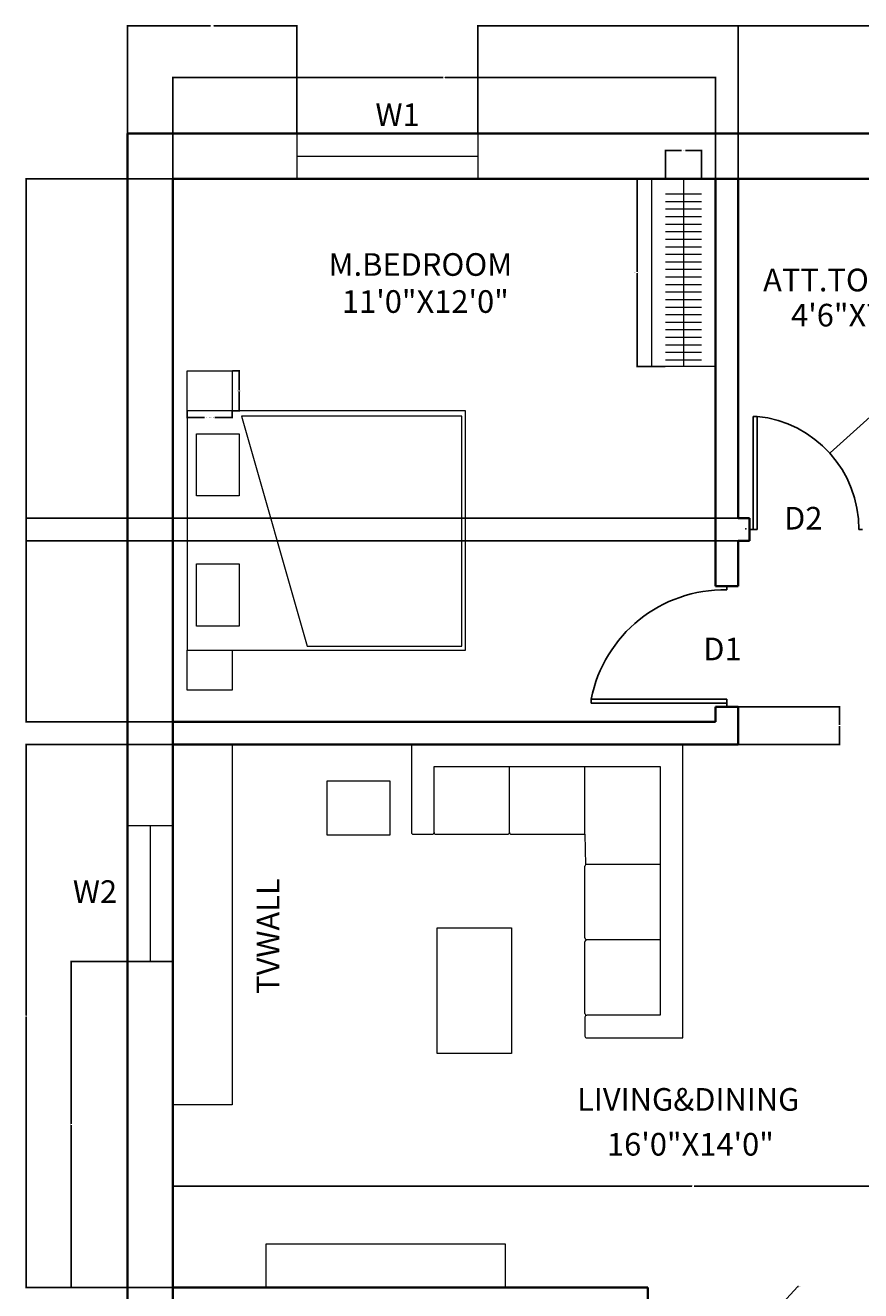
# Model space of a CAD drawing. Units: inches. Extents: x 2906 to 3403, y 1614 to 2150.
# Tile 2 of 4: x 2906 to 3127, y 1814 to 2150. Entities that reach past the tile are written whole.
import ezdxf

# ---------------------------------------------------------------- set-up
doc = ezdxf.new("R2010")
doc.units = ezdxf.units.IN
for name, color, linetype, lineweight in [('A-ANNO-DIMS', 2, 'Continuous', 18), ('A-ANNO-TEXT', 220, 'Continuous', 18), ('A-AREA-IDEN', 220, 'Continuous', 25), ('A-DOOR', 40, 'Continuous', 25), ('A-FLOR-CASE', 121, 'Continuous', 18), ('A-FURN', 121, 'Continuous', 18), ('A-GLAZ', 2, 'Continuous', 18), ('A-WALL', 191, 'Continuous', 35)]:
    doc.layers.add(name, color=color, linetype=linetype, lineweight=lineweight)
doc.styles.get("Standard").update_dxf_attribs({"font": 'arial.ttf'})
doc.dimstyles.get("Standard").update_dxf_attribs({"dimtxt": 0.18, "dimasz": 0.18, "dimexe": 0.18, "dimexo": 0.0625, "dimgap": 0.09, "dimtad": 0, "dimtih": 1, "dimtoh": 1, "dimdec": 4, "dimzin": 0, "dimdsep": 46, "dimtxsty": 'Standard', "dimcen": 0.09, "dimadec": 0, "dimazin": 0, "dimtfac": 1, "dimtdec": 4, "dimtofl": 0, "dimtmove": 0, "dimatfit": 3, "dimfxl": 1, "dimtolj": 1, "dimtzin": 0, "dimarcsym": 0})

# ---------------------------------------------------------------- blocks, each defined once
blk = doc.blocks.new('DOOR-SWING-36')
for p, q in [((36, 32), (36, 31)), ((0, 1), (0, 2)), ((0, 2), (36, 2)), ((36, 1), (0, 1)), ((36, 2), (36, 1)), ((36, 0), (36, 1))]:
    blk.add_line(p, q)
blk.add_arc((35.31, -4.99), 36, 88.9084, 168.7983)
blk = doc.blocks.new('WINDOW-48')
for p, q in [((0, 12), (0, 0)), ((48, 12), (48, 0)), ((0, 6), (48, 6))]:
    blk.add_line(p, q)
blk = doc.blocks.new('WINDOW-36')
for p, q in [((12, 36), (0, 36)), ((6, 36), (6, 0)), ((12, 0), (0, 0))]:
    blk.add_line(p, q)
blk = doc.blocks.new('WARDROBE-RAIL')
for p, q in [((4.8, 49.77), (4.8, 0)), ((0, 45.77), (9.61, 45.77)), ((0, 43.77), (9.61, 43.77)), ((0, 41.77), (9.61, 41.77)), ((0, 39.77), (9.61, 39.77)), ((0, 37.77), (9.61, 37.77)), ((0, 35.77), (9.61, 35.77)), ((0, 33.77), (9.61, 33.77)), ((0, 31.77), (9.61, 31.77)), ((0, 29.77), (9.61, 29.77)), ((0, 27.77), (9.61, 27.77)), ((0, 25.77), (9.61, 25.77)), ((0, 23.77), (9.61, 23.77)), ((0, 21.77), (9.61, 21.77)), ((0, 19.77), (9.61, 19.77)), ((0, 17.77), (9.61, 17.77)), ((0, 15.77), (9.61, 15.77)), ((0, 13.77), (9.61, 13.77)), ((0, 11.77), (9.61, 11.77)), ((0, 9.77), (9.61, 9.77)), ((0, 7.77), (9.61, 7.77)), ((0, 5.77), (9.61, 5.77)), ((0, 3.77), (9.61, 3.77)), ((0, 1.77), (9.61, 1.77))]:
    blk.add_line(p, q)
blk = doc.blocks.new('NIGHTSTAND')
blk.add_lwpolyline([(0, 10.63), (12.01, 10.63), (12.01, 0), (0, 0)], close=True)
blk = doc.blocks.new('BED-PILLOW')
blk.add_lwpolyline([(0, 16.48), (11.36, 16.48), (11.36, 0), (0, 0)], close=True)
blk = doc.blocks.new('*D14')
at = {"layer": 'A-ANNO-DIMS', "color": 0, "lineweight": -2, "transparency": 16777216}
for p, q in [((2948.43, 2047.66), (2948.43, 2045.74)), ((2960.44, 2047.66), (2960.44, 2045.74)), ((2948.61, 2045.92), (2953.06, 2045.92)), ((2960.26, 2045.92), (2955.81, 2045.92))]:
    blk.add_line(p, q, dxfattribs=at)
at = {"layer": 'A-ANNO-DIMS', "color": 0, "transparency": 16777216}
for points in [[(2948.61, 2045.95), (2948.61, 2045.89), (2948.43, 2045.92)], [(2960.26, 2045.95), (2960.26, 2045.89), (2960.44, 2045.92)]]:
    blk.add_solid(points, dxfattribs=at)
at = {"layer": 'Defpoints', "color": 0, "transparency": 16777216}
for p in [(2948.43, 2047.72), (2960.44, 2047.72), (2960.44, 2045.92)]:
    blk.add_point(p, dxfattribs=at)
at = {"layer": 'A-ANNO-DIMS', "color": 0, "transparency": 16777216, "insert": (2954.44, 2045.92), "char_height": 0.18, "attachment_point": 5}
blk.add_mtext('\\A1;NIGHTSTAND 12 TYP.', dxfattribs=at)
blk = doc.blocks.new('*D15')
at = {"layer": 'A-ANNO-DIMS', "color": 0, "lineweight": -2, "transparency": 16777216}
for p, q in [((2960.51, 2058.35), (2962.42, 2058.35)), ((2962.24, 2058.17), (2962.24, 2053.21)), ((2962.24, 2047.9), (2962.24, 2052.85)), ((2960.51, 2047.72), (2962.42, 2047.72))]:
    blk.add_line(p, q, dxfattribs=at)
at = {"layer": 'A-ANNO-DIMS', "color": 0, "transparency": 16777216}
for points in [[(2962.21, 2058.17), (2962.27, 2058.17), (2962.24, 2058.35)], [(2962.21, 2047.9), (2962.27, 2047.9), (2962.24, 2047.72)]]:
    blk.add_solid(points, dxfattribs=at)
at = {"layer": 'Defpoints', "color": 0, "transparency": 16777216}
for p in [(2960.44, 2058.35), (2962.24, 2058.35), (2960.44, 2047.72)]:
    blk.add_point(p, dxfattribs=at)
at = {"layer": 'A-ANNO-DIMS', "color": 0, "transparency": 16777216, "insert": (2962.24, 2053.03), "char_height": 0.18, "attachment_point": 5}
blk.add_mtext('\\A1;11 TYP.', dxfattribs=at)
blk = doc.blocks.new('*D30')
at = {"layer": 'A-ANNO-DIMS', "color": 0, "lineweight": -2, "transparency": 16777216}
for p, q in [((3075.27, 2109.25), (3067.69, 2109.25)), ((3067.87, 2109.07), (3067.87, 2084.55)), ((3067.87, 2059.66), (3067.87, 2084.19)), ((3075.27, 2059.48), (3067.69, 2059.48))]:
    blk.add_line(p, q, dxfattribs=at)
at = {"layer": 'A-ANNO-DIMS', "color": 0, "transparency": 16777216}
for points in [[(3067.84, 2109.07), (3067.9, 2109.07), (3067.87, 2109.25)], [(3067.84, 2059.66), (3067.9, 2059.66), (3067.87, 2059.48)]]:
    blk.add_solid(points, dxfattribs=at)
at = {"layer": 'Defpoints', "color": 0, "transparency": 16777216}
for p in [(3067.87, 2109.25), (3075.33, 2109.25), (3075.33, 2059.48)]:
    blk.add_point(p, dxfattribs=at)
at = {"layer": 'A-ANNO-DIMS', "color": 0, "transparency": 16777216, "insert": (3067.87, 2084.37), "char_height": 0.18, "attachment_point": 5}
blk.add_mtext('\\A1;RAIL 50 TYP.', dxfattribs=at)
blk = doc.blocks.new('*D31')
at = {"layer": 'A-ANNO-DIMS', "color": 0, "lineweight": -2, "transparency": 16777216}
for p, q in [((3075.33, 2109.32), (3075.33, 2116.9)), ((3075.51, 2116.72), (3079.62, 2116.72)), ((3084.76, 2116.72), (3080.66, 2116.72)), ((3084.94, 2109.32), (3084.94, 2116.9))]:
    blk.add_line(p, q, dxfattribs=at)
at = {"layer": 'A-ANNO-DIMS', "color": 0, "transparency": 16777216}
for points in [[(3075.51, 2116.75), (3075.51, 2116.69), (3075.33, 2116.72)], [(3084.76, 2116.75), (3084.76, 2116.69), (3084.94, 2116.72)]]:
    blk.add_solid(points, dxfattribs=at)
at = {"layer": 'Defpoints', "color": 0, "transparency": 16777216}
for p in [(3084.94, 2116.72), (3075.33, 2109.25), (3084.94, 2109.25)]:
    blk.add_point(p, dxfattribs=at)
at = {"layer": 'A-ANNO-DIMS', "color": 0, "transparency": 16777216, "insert": (3080.14, 2116.72), "char_height": 0.18, "attachment_point": 5}
blk.add_mtext('\\A1;10 TYP.', dxfattribs=at)
blk = doc.blocks.new('*D42')
at = {"layer": 'A-ANNO-DIMS', "color": 0, "lineweight": -2, "transparency": 16777216}
for p, q in [((2932.63, 2121.32), (2932.63, 2149.96)), ((2932.81, 2149.78), (2954.7, 2149.78)), ((2977.39, 2149.78), (2955.5, 2149.78)), ((2977.57, 2121.32), (2977.57, 2149.96))]:
    blk.add_line(p, q, dxfattribs=at)
at = {"layer": 'A-ANNO-DIMS', "color": 0, "transparency": 16777216}
for points in [[(2932.81, 2149.81), (2932.81, 2149.75), (2932.63, 2149.78)], [(2977.39, 2149.81), (2977.39, 2149.75), (2977.57, 2149.78)]]:
    blk.add_solid(points, dxfattribs=at)
at = {"layer": 'Defpoints', "color": 0, "transparency": 16777216}
for p in [(2977.57, 2149.78), (2932.63, 2121.25), (2977.57, 2121.25)]:
    blk.add_point(p, dxfattribs=at)
at = {"layer": 'A-ANNO-DIMS', "color": 0, "transparency": 16777216, "insert": (2955.1, 2149.78), "char_height": 0.18, "attachment_point": 5}
blk.add_mtext('\\A1;44.93', dxfattribs=at)
blk = doc.blocks.new('*D43')
at = {"layer": 'A-ANNO-DIMS', "color": 0, "lineweight": -2, "transparency": 16777216}
for p, q in [((3025.57, 2121.32), (3025.57, 2149.96)), ((3025.75, 2149.78), (3108.75, 2149.78)), ((3192.49, 2149.78), (3109.49, 2149.78)), ((3192.67, 2121.32), (3192.67, 2149.96))]:
    blk.add_line(p, q, dxfattribs=at)
at = {"layer": 'A-ANNO-DIMS', "color": 0, "transparency": 16777216}
for points in [[(3025.75, 2149.81), (3025.75, 2149.75), (3025.57, 2149.78)], [(3192.49, 2149.81), (3192.49, 2149.75), (3192.67, 2149.78)]]:
    blk.add_solid(points, dxfattribs=at)
at = {"layer": 'Defpoints', "color": 0, "transparency": 16777216}
for p in [(3192.67, 2149.78), (3025.57, 2121.25), (3192.67, 2121.25)]:
    blk.add_point(p, dxfattribs=at)
at = {"layer": 'A-ANNO-DIMS', "color": 0, "transparency": 16777216, "insert": (3109.12, 2149.78), "char_height": 0.18, "attachment_point": 5}
blk.add_mtext('\\A1;167.1', dxfattribs=at)
blk = doc.blocks.new('*D45')
at = {"layer": 'A-ANNO-DIMS', "color": 0, "lineweight": -2, "transparency": 16777216}
for p, q in [((2944.63, 2109.32), (2944.63, 2136.33)), ((2944.81, 2136.15), (3016.35, 2136.15)), ((3088.45, 2136.15), (3016.91, 2136.15)), ((3088.63, 2109.32), (3088.63, 2136.33))]:
    blk.add_line(p, q, dxfattribs=at)
at = {"layer": 'A-ANNO-DIMS', "color": 0, "transparency": 16777216}
for points in [[(2944.81, 2136.18), (2944.81, 2136.12), (2944.63, 2136.15)], [(3088.45, 2136.18), (3088.45, 2136.12), (3088.63, 2136.15)]]:
    blk.add_solid(points, dxfattribs=at)
at = {"layer": 'Defpoints', "color": 0, "transparency": 16777216}
for p in [(3088.63, 2136.15), (2944.63, 2109.25), (3088.63, 2109.25)]:
    blk.add_point(p, dxfattribs=at)
at = {"layer": 'A-ANNO-DIMS', "color": 0, "transparency": 16777216, "insert": (3016.63, 2136.15), "char_height": 0.18, "attachment_point": 5}
blk.add_mtext('\\A1;144', dxfattribs=at)
blk = doc.blocks.new('*D46')
at = {"layer": 'A-ANNO-DIMS', "color": 0, "lineweight": -2, "transparency": 16777216}
for p, q in [((3094.63, 2109.32), (3094.63, 2149.96)), ((3094.81, 2149.78), (3124.41, 2149.78)), ((3154.45, 2149.78), (3124.85, 2149.78)), ((3154.63, 2109.32), (3154.63, 2149.96))]:
    blk.add_line(p, q, dxfattribs=at)
at = {"layer": 'A-ANNO-DIMS', "color": 0, "transparency": 16777216}
for points in [[(3094.81, 2149.81), (3094.81, 2149.75), (3094.63, 2149.78)], [(3154.45, 2149.81), (3154.45, 2149.75), (3154.63, 2149.78)]]:
    blk.add_solid(points, dxfattribs=at)
at = {"layer": 'Defpoints', "color": 0, "transparency": 16777216}
for p in [(3154.63, 2149.78), (3094.63, 2109.25), (3154.63, 2109.25)]:
    blk.add_point(p, dxfattribs=at)
at = {"layer": 'A-ANNO-DIMS', "color": 0, "transparency": 16777216, "insert": (3124.63, 2149.78), "char_height": 0.18, "attachment_point": 5}
blk.add_mtext('\\A1;60', dxfattribs=at)
blk = doc.blocks.new('*D49')
at = {"layer": 'A-ANNO-DIMS', "color": 0, "lineweight": -2, "transparency": 16777216}
for p, q in [((2944.57, 1959.25), (2905.55, 1959.25)), ((2905.73, 1959.07), (2905.73, 1887.43)), ((2905.73, 1815.43), (2905.73, 1887.07)), ((2944.57, 1815.25), (2905.55, 1815.25))]:
    blk.add_line(p, q, dxfattribs=at)
at = {"layer": 'A-ANNO-DIMS', "color": 0, "transparency": 16777216}
for points in [[(2905.7, 1959.07), (2905.76, 1959.07), (2905.73, 1959.25)], [(2905.7, 1815.43), (2905.76, 1815.43), (2905.73, 1815.25)]]:
    blk.add_solid(points, dxfattribs=at)
at = {"layer": 'Defpoints', "color": 0, "transparency": 16777216}
for p in [(2905.73, 1959.25), (2944.63, 1959.25), (2944.63, 1815.25)]:
    blk.add_point(p, dxfattribs=at)
at = {"layer": 'A-ANNO-DIMS', "color": 0, "transparency": 16777216, "insert": (2905.73, 1887.25), "char_height": 0.18, "attachment_point": 5}
blk.add_mtext('\\A1;144', dxfattribs=at)
blk = doc.blocks.new('*D50')
at = {"layer": 'A-ANNO-DIMS', "color": 0, "lineweight": -2, "transparency": 16777216}
for p, q in [((2944.57, 2109.25), (2905.55, 2109.25)), ((2905.73, 2109.07), (2905.73, 2037.43)), ((2905.73, 1965.43), (2905.73, 2037.07)), ((2944.57, 1965.25), (2905.55, 1965.25))]:
    blk.add_line(p, q, dxfattribs=at)
at = {"layer": 'A-ANNO-DIMS', "color": 0, "transparency": 16777216}
for points in [[(2905.7, 2109.07), (2905.76, 2109.07), (2905.73, 2109.25)], [(2905.7, 1965.43), (2905.76, 1965.43), (2905.73, 1965.25)]]:
    blk.add_solid(points, dxfattribs=at)
at = {"layer": 'Defpoints', "color": 0, "transparency": 16777216}
for p in [(2905.73, 2109.25), (2944.63, 2109.25), (2944.63, 1965.25)]:
    blk.add_point(p, dxfattribs=at)
at = {"layer": 'A-ANNO-DIMS', "color": 0, "transparency": 16777216, "insert": (2905.73, 2037.25), "char_height": 0.18, "attachment_point": 5}
blk.add_mtext('\\A1;144', dxfattribs=at)
blk = doc.blocks.new('*D51')
at = {"layer": 'A-ANNO-DIMS', "color": 0, "lineweight": -2, "transparency": 16777216}
for p, q in [((2944.57, 1901.7), (2917.55, 1901.7)), ((2917.73, 1901.52), (2917.73, 1858.66)), ((2917.73, 1815.43), (2917.73, 1858.29)), ((2944.57, 1815.25), (2917.55, 1815.25))]:
    blk.add_line(p, q, dxfattribs=at)
at = {"layer": 'A-ANNO-DIMS', "color": 0, "transparency": 16777216}
for points in [[(2917.7, 1901.52), (2917.76, 1901.52), (2917.73, 1901.7)], [(2917.7, 1815.43), (2917.76, 1815.43), (2917.73, 1815.25)]]:
    blk.add_solid(points, dxfattribs=at)
at = {"layer": 'Defpoints', "color": 0, "transparency": 16777216}
for p in [(2917.73, 1901.7), (2944.63, 1901.7), (2944.63, 1815.25)]:
    blk.add_point(p, dxfattribs=at)
at = {"layer": 'A-ANNO-DIMS', "color": 0, "transparency": 16777216, "insert": (2917.73, 1858.48), "char_height": 0.18, "attachment_point": 5}
blk.add_mtext('\\A1;86.44', dxfattribs=at)
blk = doc.blocks.new('*D65')
at = {"layer": 'A-ANNO-DIMS', "color": 0, "lineweight": -2, "transparency": 16777216}
for p, q in [((2944.63, 1815.32), (2944.63, 1842.33)), ((2944.81, 1842.15), (3082.34, 1842.15)), ((3220.45, 1842.15), (3082.92, 1842.15)), ((3220.63, 1815.32), (3220.63, 1842.33))]:
    blk.add_line(p, q, dxfattribs=at)
at = {"layer": 'A-ANNO-DIMS', "color": 0, "transparency": 16777216}
for points in [[(2944.81, 1842.18), (2944.81, 1842.12), (2944.63, 1842.15)], [(3220.45, 1842.18), (3220.45, 1842.12), (3220.63, 1842.15)]]:
    blk.add_solid(points, dxfattribs=at)
at = {"layer": 'Defpoints', "color": 0, "transparency": 16777216}
for p in [(3220.63, 1842.15), (2944.63, 1815.25), (3220.63, 1815.25)]:
    blk.add_point(p, dxfattribs=at)
at = {"layer": 'A-ANNO-DIMS', "color": 0, "transparency": 16777216, "insert": (3082.63, 1842.15), "char_height": 0.18, "attachment_point": 5}
blk.add_mtext('\\A1;276', dxfattribs=at)
blk = doc.blocks.new('*D71')
at = {"layer": 'A-ANNO-DIMS', "color": 0, "lineweight": -2, "transparency": 16777216}
for p, q in [((3094.7, 1969.25), (3121.71, 1969.25)), ((3121.53, 1969.07), (3121.53, 1964.44)), ((3121.53, 1959.43), (3121.53, 1964.07)), ((3094.7, 1959.25), (3121.71, 1959.25))]:
    blk.add_line(p, q, dxfattribs=at)
at = {"layer": 'A-ANNO-DIMS', "color": 0, "transparency": 16777216}
for points in [[(3121.5, 1969.07), (3121.56, 1969.07), (3121.53, 1969.25)], [(3121.5, 1959.43), (3121.56, 1959.43), (3121.53, 1959.25)]]:
    blk.add_solid(points, dxfattribs=at)
at = {"layer": 'Defpoints', "color": 0, "transparency": 16777216}
for p in [(3094.63, 1969.25), (3094.63, 1959.25), (3121.53, 1959.25)]:
    blk.add_point(p, dxfattribs=at)
at = {"layer": 'A-ANNO-DIMS', "color": 0, "transparency": 16777216, "insert": (3121.53, 1964.25), "char_height": 0.18, "attachment_point": 5}
blk.add_mtext('\\A1;10', dxfattribs=at)
blk = doc.blocks.new('*D73')
at = {"layer": 'A-ANNO-DIMS', "color": 0, "lineweight": -2, "transparency": 16777216}
for p, q in [((3094.57, 2109.25), (2905.55, 2109.25)), ((2905.73, 2109.07), (2905.73, 2064.44)), ((2905.73, 2019.43), (2905.73, 2064.07)), ((3094.57, 2019.25), (2905.55, 2019.25))]:
    blk.add_line(p, q, dxfattribs=at)
at = {"layer": 'A-ANNO-DIMS', "color": 0, "transparency": 16777216}
for points in [[(2905.7, 2109.07), (2905.76, 2109.07), (2905.73, 2109.25)], [(2905.7, 2019.43), (2905.76, 2019.43), (2905.73, 2019.25)]]:
    blk.add_solid(points, dxfattribs=at)
at = {"layer": 'Defpoints', "color": 0, "transparency": 16777216}
for p in [(2905.73, 2109.25), (3094.63, 2109.25), (3094.63, 2019.25)]:
    blk.add_point(p, dxfattribs=at)
at = {"layer": 'A-ANNO-DIMS', "color": 0, "transparency": 16777216, "insert": (2905.73, 2064.25), "char_height": 0.18, "attachment_point": 5}
blk.add_mtext('\\A1;90', dxfattribs=at)
blk = doc.blocks.new('*D74')
at = {"layer": 'A-ANNO-DIMS', "color": 0, "lineweight": -2, "transparency": 16777216}
for p, q in [((3094.57, 2019.25), (2905.55, 2019.25)), ((2905.73, 2019.07), (2905.73, 2016.44)), ((3094.57, 2013.25), (2905.55, 2013.25)), ((2905.73, 2013.43), (2905.73, 2016.07))]:
    blk.add_line(p, q, dxfattribs=at)
at = {"layer": 'A-ANNO-DIMS', "color": 0, "transparency": 16777216}
for points in [[(2905.7, 2019.07), (2905.76, 2019.07), (2905.73, 2019.25)], [(2905.7, 2013.43), (2905.76, 2013.43), (2905.73, 2013.25)]]:
    blk.add_solid(points, dxfattribs=at)
at = {"layer": 'Defpoints', "color": 0, "transparency": 16777216}
for p in [(2905.73, 2019.25), (3094.63, 2019.25), (3094.63, 2013.25)]:
    blk.add_point(p, dxfattribs=at)
at = {"layer": 'A-ANNO-DIMS', "color": 0, "transparency": 16777216, "insert": (2905.73, 2016.25), "char_height": 0.18, "attachment_point": 5}
blk.add_mtext('\\A1;6', dxfattribs=at)
blk = doc.blocks.new('*D80')
at = {"layer": 'A-ANNO-DIMS', "color": 0, "lineweight": -2, "transparency": 16777216}
for p, q in [((3110.47, 1815.5), (3093.44, 1797.16)), ((3110.65, 1815.5), (3110.47, 1815.5)), ((3064.65, 1766.25), (3064.83, 1766.25)), ((3064.74, 1766.16), (3064.74, 1766.34))]:
    blk.add_line(p, q, dxfattribs=at)
at = {"layer": 'A-ANNO-DIMS', "color": 0, "transparency": 16777216}
blk.add_solid([(3093.42, 1797.18), (3093.46, 1797.14), (3093.32, 1797.03)], dxfattribs=at)
at = {"layer": 'Defpoints', "color": 0, "transparency": 16777216}
for p in [(3093.32, 1797.03), (3064.74, 1766.25)]:
    blk.add_point(p, dxfattribs=at)
at = {"layer": 'A-ANNO-DIMS', "color": 0, "transparency": 16777216, "insert": (3110.95, 1815.5), "char_height": 0.18, "attachment_point": 5}
blk.add_mtext('\\A1;R42', dxfattribs=at)
blk = doc.blocks.new('*D82')
at = {"layer": 'A-ANNO-DIMS', "color": 0, "lineweight": -2, "transparency": 16777216}
for p, q in [((3132.31, 2048.51), (3119.07, 2036.59)), ((3132.49, 2048.51), (3132.31, 2048.51)), ((3096.54, 2016.4), (3096.72, 2016.4)), ((3096.63, 2016.31), (3096.63, 2016.49))]:
    blk.add_line(p, q, dxfattribs=at)
at = {"layer": 'A-ANNO-DIMS', "color": 0, "transparency": 16777216}
blk.add_solid([(3119.05, 2036.62), (3119.09, 2036.57), (3118.93, 2036.47)], dxfattribs=at)
at = {"layer": 'Defpoints', "color": 0, "transparency": 16777216}
for p in [(3118.93, 2036.47), (3096.63, 2016.4)]:
    blk.add_point(p, dxfattribs=at)
at = {"layer": 'A-ANNO-DIMS', "color": 0, "transparency": 16777216, "insert": (3132.8, 2048.51), "char_height": 0.18, "attachment_point": 5}
blk.add_mtext('\\A1;R30', dxfattribs=at)

msp = doc.modelspace()

# ---------------------------------------------------------------- linework, layer by layer
at = {"layer": 'A-DOOR'}
for p, q in [((3098.6325, 2016.254), (3098.6325, 2046.254)), ((3098.6325, 2046.254), (3099.6325, 2046.254)), ((3099.6325, 2046.254), (3099.6325, 2016.254)), ((3097.6325, 2016.254), (3098.6325, 2016.254)), ((3099.6325, 2016.254), (3098.6325, 2016.254)), ((3127.6325, 2016.254), (3126.6325, 2016.254))]:
    msp.add_line(p, q, dxfattribs=at)
msp.add_arc((3096.6329, 2016.4043), 30, 359.712872, 84.261553, dxfattribs=at)
at = {"layer": 'A-FLOR-CASE'}
for p, q in [((3071.6325, 2109.254), (3088.6325, 2109.254)), ((3071.6325, 2109.254), (3071.6325, 2059.4818)), ((3088.6325, 2059.4818), (3071.6325, 2059.4818)), ((2960.435, 1959.254), (2960.435, 1863.6695)), ((2960.435, 1863.6695), (2944.6325, 1863.6695)), ((2969.4494, 1815.254), (2969.4494, 1826.8243)), ((2969.4494, 1826.8243), (3032.8231, 1826.8243)), ((3032.8231, 1826.8243), (3032.8231, 1815.254))]:
    msp.add_line(p, q, dxfattribs=at)
at = {"layer": 'A-FURN'}
for p, q in [((3021.3378, 2046.2873), (2962.8957, 2046.2873)), ((2962.8957, 2046.2873), (2980.3378, 1985.2873)), ((3021.3378, 1985.2873), (3021.3378, 2046.2873)), ((2980.3378, 1985.2873), (3021.3378, 1985.2873)), ((3007.9653, 1959.254), (3007.9653, 1935.9495)), ((3079.9653, 1959.254), (3007.9653, 1959.254)), ((3079.9653, 1881.4495), (3079.9653, 1959.254)), ((3013.9653, 1935.9495), (3013.9653, 1953.4495)), ((3013.9653, 1953.4495), (3073.9653, 1953.4495)), ((3033.9653, 1935.9495), (3033.9653, 1953.4495)), ((3053.9653, 1935.4495), (3053.9653, 1953.4495)), ((3073.9653, 1953.4495), (3073.9653, 1887.4495)), ((3008.4653, 1935.4495), (3013.4653, 1935.4495)), ((3013.9653, 1935.9495), (3013.9653, 1935.9495)), ((3014.4653, 1935.4495), (3033.4653, 1935.4495)), ((3033.9653, 1935.9495), (3033.9653, 1935.9495)), ((3034.4653, 1935.4495), (3053.9653, 1935.4495)), ((3053.9653, 1935.4495), (3054.1118, 1927.3031)), ((3053.9653, 1907.9495), (3053.9653, 1926.9495)), ((3073.9653, 1927.4495), (3054.4653, 1927.4495)), ((3053.9653, 1887.9495), (3053.9653, 1906.9495)), ((3073.9653, 1907.4495), (3054.4653, 1907.4495)), ((3054.4653, 1907.4495), (3054.4653, 1907.4495)), ((3053.9653, 1886.9495), (3053.9653, 1881.9495)), ((3073.9653, 1887.4495), (3054.4653, 1887.4495)), ((3054.4653, 1887.4495), (3054.4653, 1887.4495)), ((3054.4653, 1881.4495), (3079.9653, 1881.4495))]:
    msp.add_line(p, q, dxfattribs=at)
for points in [[(2948.4332, 1984.2873), (3022.3293, 1984.2873), (3022.3293, 2047.7187), (2948.4332, 2047.7187)], [(2985.566, 1949.6418), (3002.2289, 1949.6418), (3002.2289, 1935.1766), (2985.566, 1935.1766)], [(3014.7944, 1910.6131), (3034.4621, 1910.6131), (3034.4621, 1877.3159), (3014.7944, 1877.3159)]]:
    msp.add_lwpolyline(points, close=True, dxfattribs=at)
for centre, start, end in [((3008.4653, 1935.9495), 180, 270), ((3013.4653, 1935.9495), 270, 0), ((3014.4653, 1935.9495), 180, 270), ((3033.4653, 1935.9495), 270, 0), ((3034.4653, 1935.9495), 180, 270), ((3054.4653, 1926.9495), 90, 180), ((3054.4653, 1907.9495), 180, 270), ((3054.4653, 1906.9495), 90, 180), ((3054.4653, 1887.9495), 180, 270), ((3054.4653, 1886.9495), 90, 180), ((3054.4653, 1881.9495), 180, 270)]:
    msp.add_arc(centre, 0.5, start, end, dxfattribs=at)
at = {"layer": 'A-WALL'}
for p, q in [((2944.6325, 2109.254), (3280.6325, 2109.254)), ((2944.6325, 1809.254), (2944.6325, 2109.254)), ((3088.6325, 2001.254), (3088.6325, 2109.254)), ((3094.6325, 2019.254), (3094.6325, 2109.254)), ((3094.6325, 2019.254), (3097.6325, 2019.254)), ((3097.6325, 2013.254), (3097.6325, 2019.254)), ((3094.6325, 2013.254), (3097.6325, 2013.254)), ((3094.6325, 2001.254), (3094.6325, 2013.254)), ((3088.6325, 2001.254), (3094.6325, 2001.254)), ((3088.6325, 1965.254), (3088.6325, 1969.254)), ((3088.6325, 1969.254), (3094.6325, 1969.254)), ((3094.6325, 1969.254), (3094.6325, 1965.254)), ((2944.6325, 1965.254), (3088.6325, 1965.254)), ((3094.6325, 1959.254), (3094.6325, 1965.254)), ((2944.6325, 1959.254), (3094.6325, 1959.254)), ((2944.6325, 1815.254), (3070.6325, 1815.254)), ((3070.6325, 1809.254), (3070.6325, 1815.254))]:
    msp.add_line(p, q, dxfattribs=at)
msp.add_lwpolyline([(3022.1668, 1641.254), (2932.6325, 1641.254), (2932.6325, 2121.254), (3292.6325, 2121.254), (3292.6325, 1689.254)], dxfattribs=at)

# ---------------------------------------------------------------- block references
at = {"layer": 'A-DOOR'}
msp.add_blockref('DOOR-SWING-36', (3055.633, 1969.254), dxfattribs=at)
at = {"layer": 'A-FLOR-CASE'}
msp.add_blockref('WARDROBE-RAIL', (3075.334, 2059.482), dxfattribs=at)
at = {"layer": 'A-FURN'}
for name, p in [('NIGHTSTAND', (2948.433, 2047.7191)), ('BED-PILLOW', (2950.931, 2025.159)), ('BED-PILLOW', (2950.931, 1990.6499)), ('NIGHTSTAND', (2948.433, 1973.659))]:
    msp.add_blockref(name, p, dxfattribs=at)
at = {"layer": 'A-GLAZ'}
for name, p in [('WINDOW-48', (2977.566, 2109.254)), ('WINDOW-36', (2932.633, 1901.696))]:
    msp.add_blockref(name, p, dxfattribs=at)

# ---------------------------------------------------------------- texts
at = {"layer": 'A-ANNO-TEXT'}
for tag, p in [('W1', (2998.406, 2123.2386)), ('D2', (3106.8, 2016.254)), ('D1', (3085.3604, 1981.5794)), ('W2', (2918.146, 1917.2392))]:
    msp.add_attdef(tag, p, '', height=6, dxfattribs=at)
msp.add_attdef('TVWALL', (2972.9207, 1893.1123), '', height=6, rotation=90, dxfattribs=at)
at = {"layer": 'A-AREA-IDEN'}
for tag, p in [('M.BEDROOM', (2985.961, 2083.5309)), ('ATT.TOILET', (3101.2536, 2079.4131)), ('11\'0"X12\'0"', (2989.5237, 2073.7127)), ('4\'6"X7\'6"', (3108.6552, 2070.1006)), ('LIVING&DINING', (3051.8934, 1862.1429)), ('16\'0"X14\'0"', (3059.8362, 1850.239))]:
    msp.add_attdef(tag, p, '', height=6, dxfattribs=at)

# ---------------------------------------------------------------- dimensions: what is measured, and where the dimension line sits
at = {"layer": 'A-ANNO-DIMS'}
for base, p1, p2, override, picture, middle in [((2977.5663, 2149.7771), (2932.6325, 2121.254), (2977.5663, 2121.254), {"dimdec": 2, "dimlfac": 1, "dimrnd": 0, "dimzin": 0, "dimdsep": 46, "dimlunit": 2}, '*D42', (2955.0994, 2149.7771)), ((3192.6748, 2149.7771), (3025.5663, 2121.254), (3192.6748, 2121.254), {"dimdec": 1, "dimlfac": 1, "dimrnd": 0, "dimzin": 0, "dimdsep": 46, "dimlunit": 2}, '*D43', (3109.1205, 2149.7771)), ((3154.6325, 2149.7771), (3094.6325, 2109.254), (3154.6325, 2109.254), {"dimdec": 0, "dimlfac": 1, "dimrnd": 0, "dimzin": 0, "dimdsep": 46, "dimlunit": 2}, '*D46', (3124.6325, 2149.7771)), ((3088.6325, 2136.154), (2944.6325, 2109.254), (3088.6325, 2109.254), {"dimdec": 0, "dimlfac": 1, "dimrnd": 0, "dimzin": 0, "dimdsep": 46, "dimlunit": 2}, '*D45', (3016.6325, 2136.154)), ((3220.6325, 1842.154), (2944.6325, 1815.254), (3220.6325, 1815.254), {"dimdec": 0, "dimlfac": 1, "dimrnd": 0, "dimzin": 0, "dimdsep": 46, "dimlunit": 2}, '*D65', (3082.6325, 1842.154))]:
    dim = msp.add_linear_dim(base=base, p1=p1, p2=p2, dimstyle='Standard', override=override, dxfattribs=at)
    dim.commit()
    dim.dimension.update_dxf_attribs({"geometry": picture, "text_midpoint": middle})
for base, p1, p2, text, picture, middle in [((3084.9396, 2116.7198), (3075.3336, 2109.254), (3084.9396, 2109.254), '<> TYP.', '*D31', (3080.1366, 2116.7198)), ((2960.443, 2045.9172), (2948.4332, 2047.7187), (2960.443, 2047.7187), 'NIGHTSTAND <> TYP.', '*D14', (2954.4381, 2045.9172))]:
    dim = msp.add_linear_dim(base=base, p1=p1, p2=p2, text=text, dimstyle='Standard', override={"dimdec": 0, "dimlfac": 1, "dimrnd": 0, "dimzin": 0, "dimdsep": 46, "dimlunit": 2}, dxfattribs=at)
    dim.commit()
    dim.dimension.update_dxf_attribs({"geometry": picture, "text_midpoint": middle})
for base, p1, p2, angle, override, picture, middle in [((2905.7325, 2109.254), (2944.6325, 1965.254), (2944.6325, 2109.254), 90, {"dimdec": 0, "dimlfac": 1, "dimrnd": 0, "dimzin": 0, "dimdsep": 46, "dimlunit": 2}, '*D50', (2905.7325, 2037.254)), ((2905.7325, 2109.254), (3094.6325, 2019.254), (3094.6325, 2109.254), 90, {"dimdec": 0, "dimlfac": 1, "dimrnd": 0, "dimzin": 0, "dimdsep": 46, "dimlunit": 2}, '*D73', (2905.7325, 2064.254)), ((2905.7325, 2019.254), (3094.6325, 2013.254), (3094.6325, 2019.254), 90, {"dimdec": 0, "dimlfac": 1, "dimrnd": 0, "dimzin": 0, "dimdsep": 46, "dimlunit": 2}, '*D74', (2905.7325, 2016.254)), ((3121.5325, 1959.254), (3094.6325, 1969.254), (3094.6325, 1959.254), 270, {"dimdec": 0, "dimlfac": 1, "dimrnd": 0, "dimzin": 0, "dimdsep": 46, "dimlunit": 2}, '*D71', (3121.5325, 1964.254)), ((2905.7325, 1959.254), (2944.6325, 1815.254), (2944.6325, 1959.254), 90, {"dimdec": 0, "dimlfac": 1, "dimrnd": 0, "dimzin": 0, "dimdsep": 46, "dimlunit": 2}, '*D49', (2905.7325, 1887.254)), ((2917.7325, 1901.6965), (2944.6325, 1815.254), (2944.6325, 1901.6965), 90, {"dimdec": 2, "dimlfac": 1, "dimrnd": 0, "dimzin": 0, "dimdsep": 46, "dimlunit": 2}, '*D51', (2917.7325, 1858.4752))]:
    dim = msp.add_linear_dim(base=base, p1=p1, p2=p2, angle=angle, dimstyle='Standard', override=override, dxfattribs=at)
    dim.commit()
    dim.dimension.update_dxf_attribs({"geometry": picture, "text_midpoint": middle})
for base, p1, p2, text, picture, middle in [((3067.8678, 2109.254), (3075.3336, 2059.4818), (3075.3336, 2109.254), 'RAIL <> TYP.', '*D30', (3067.8678, 2084.3679)), ((2962.2445, 2058.3474), (2960.443, 2047.7187), (2960.443, 2058.3474), '<> TYP.', '*D15', (2962.2445, 2053.0331))]:
    dim = msp.add_linear_dim(base=base, p1=p1, p2=p2, angle=90, text=text, dimstyle='Standard', override={"dimdec": 0, "dimlfac": 1, "dimrnd": 0, "dimzin": 0, "dimdsep": 46, "dimlunit": 2}, dxfattribs=at)
    dim.commit()
    dim.dimension.update_dxf_attribs({"geometry": picture, "text_midpoint": middle})
for center, mpoint, picture, middle in [((3096.6329, 2016.4043), (3118.932, 2036.473), '*D82', (3132.7962, 2048.5142)), ((3064.7398, 1766.2541), (3093.3191, 1797.0311), '*D80', (3110.9508, 1815.4973))]:
    dim = msp.add_radius_dim(center=center, mpoint=mpoint, dimstyle='Standard', override={"dimdec": 0, "dimlfac": 1, "dimrnd": 0, "dimzin": 0, "dimdsep": 46, "dimlunit": 2}, dxfattribs=at)
    dim.commit()
    dim.dimension.update_dxf_attribs({"geometry": picture, "text_midpoint": middle, "dimtype": 164})

doc.saveas('drawing.dxf')
